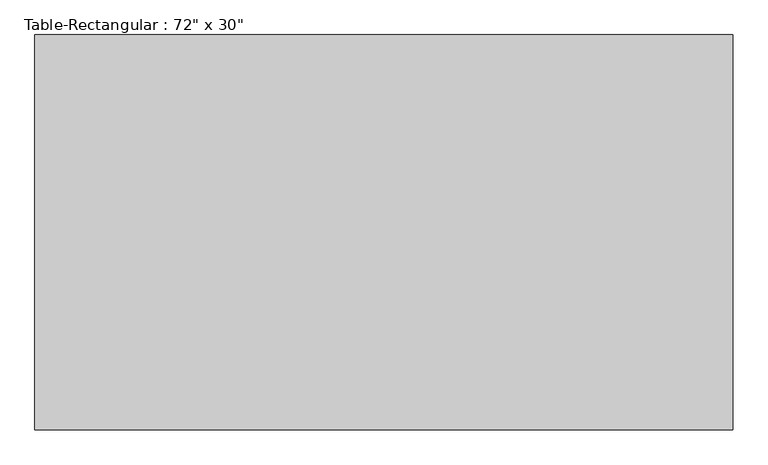
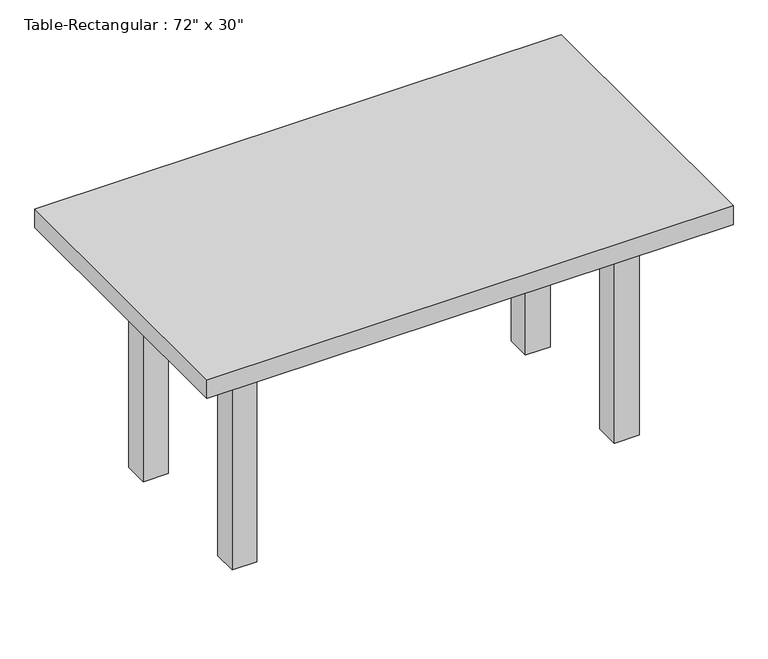
"""IFC4 building model written with IfcOpenShell, lengths in millimetres: furniture geometry."""

from ifc_helpers import new_model, si_unit, frame, origin, origin_with_axes, place, context, project, spatial, polyline, outline, extrude, source, transform, mapped, element, save


def furniture_48e8c7c4(model_context):
    return source(origin(), model_context, "Body", "SweptSolid", [
        extrude(outline(polyline([(457.2, 190.5), (457.2, 165.1), (-457.2, 165.1), (-457.2, 190.5), (457.2, 190.5)])), frame((0.0, 0.0, 508.0), z_axis=(0.0, 0.0, 1.0), x_axis=(1.0, 0.0, 0.0)), (0.0, 0.0, 1.0), 101.6),
        extrude(outline(polyline([(457.2, -190.5), (-457.2, -190.5), (-457.2, -165.1), (457.2, -165.1), (457.2, -190.5)])), frame((0.0, 0.0, 508.0), z_axis=(0.0, 0.0, 1.0), x_axis=(1.0, 0.0, 0.0)), (0.0, 0.0, 1.0), 101.6),
        extrude(outline(polyline([(-469.9, -165.1), (-495.3, -165.1), (-495.3, 165.1), (-469.9, 165.1), (-469.9, -165.1)])), frame((0.0, 0.0, 508.0), z_axis=(0.0, 0.0, 1.0), x_axis=(1.0, 0.0, 0.0)), (0.0, 0.0, 1.0), 101.6),
        extrude(outline(polyline([(469.9, -165.1), (469.9, 165.1), (495.3, 165.1), (495.3, -165.1), (469.9, -165.1)])), frame((0.0, 0.0, 508.0), z_axis=(0.0, 0.0, 1.0), x_axis=(1.0, 0.0, 0.0)), (0.0, 0.0, 1.0), 101.6),
        extrude(outline(polyline([(673.1, 381.0), (673.1, -381.0), (-673.1, -381.0), (-673.1, 381.0), (673.1, 381.0)])), frame((0.0, 0.0, 609.6), z_axis=(0.0, 0.0, 1.0), x_axis=(1.0, 0.0, 0.0)), (0.0, 0.0, 1.0), 50.8),
        extrude(outline(polyline([(-457.2, 228.6), (-457.2, 165.1), (-520.7, 165.1), (-520.7, 228.6), (-457.2, 228.6)])), origin_with_axes(), (0.0, 0.0, 1.0), 609.6),
        extrude(outline(polyline([(457.2, 228.6), (520.7, 228.6), (520.7, 165.1), (457.2, 165.1), (457.2, 228.6)])), origin_with_axes(), (0.0, 0.0, 1.0), 609.6),
        extrude(outline(polyline([(-457.2, -228.6), (-520.7, -228.6), (-520.7, -165.1), (-457.2, -165.1), (-457.2, -228.6)])), origin_with_axes(), (0.0, 0.0, 1.0), 609.6),
        extrude(outline(polyline([(457.2, -228.6), (457.2, -165.1), (520.7, -165.1), (520.7, -228.6), (457.2, -228.6)])), origin_with_axes(), (0.0, 0.0, 1.0), 609.6),
    ])


if __name__ == "__main__":
    model = new_model("IFC4")
    model_context = context("Model", 3, world=origin())
    ifc_project = project(units=[si_unit("LENGTHUNIT", "METRE", prefix="MILLI")], contexts=[model_context])
    site = spatial("IfcSite", under=ifc_project)
    building = spatial("IfcBuilding", under=site)
    placement = place(None, origin())
    furniture_shape = furniture_48e8c7c4(model_context)
    element("IfcFurniture", 1, ObjectType="Table-Rectangular : 72\" x 30\"", at=placement, inside=building, context=model_context, shape_type="MappedRepresentation", body=[
        mapped(furniture_shape, transform((0.0, 0.0, 0.0), x_axis=(1.0, 0.0, 0.0), y_axis=(0.0, 1.0, 0.0), z_axis=(0.0, 0.0, 1.0))),
    ])
    save(model, "model.ifc")

# Revit data of these elements
# Type "Table-Rectangular : 72\" x 30\""
#   Assembly Code = "E2020200"
#   Height = 2' - 2"
#   Length = 4' - 5"
#   Width = 2' - 6"
#   Base Material = Birch
#   Top Material = Birch
#   Default Elevation = 0
# Element 1 (IfcFurniture, "Table-Rectangular : 72\" x 30\"")
#   Materials on its faces: "Birch"
# Materials
#   "Birch": class "Wood", colour RGB 210 159 95, transparency 0, Description = "Betula Alleghaniensis", Cost = 0
